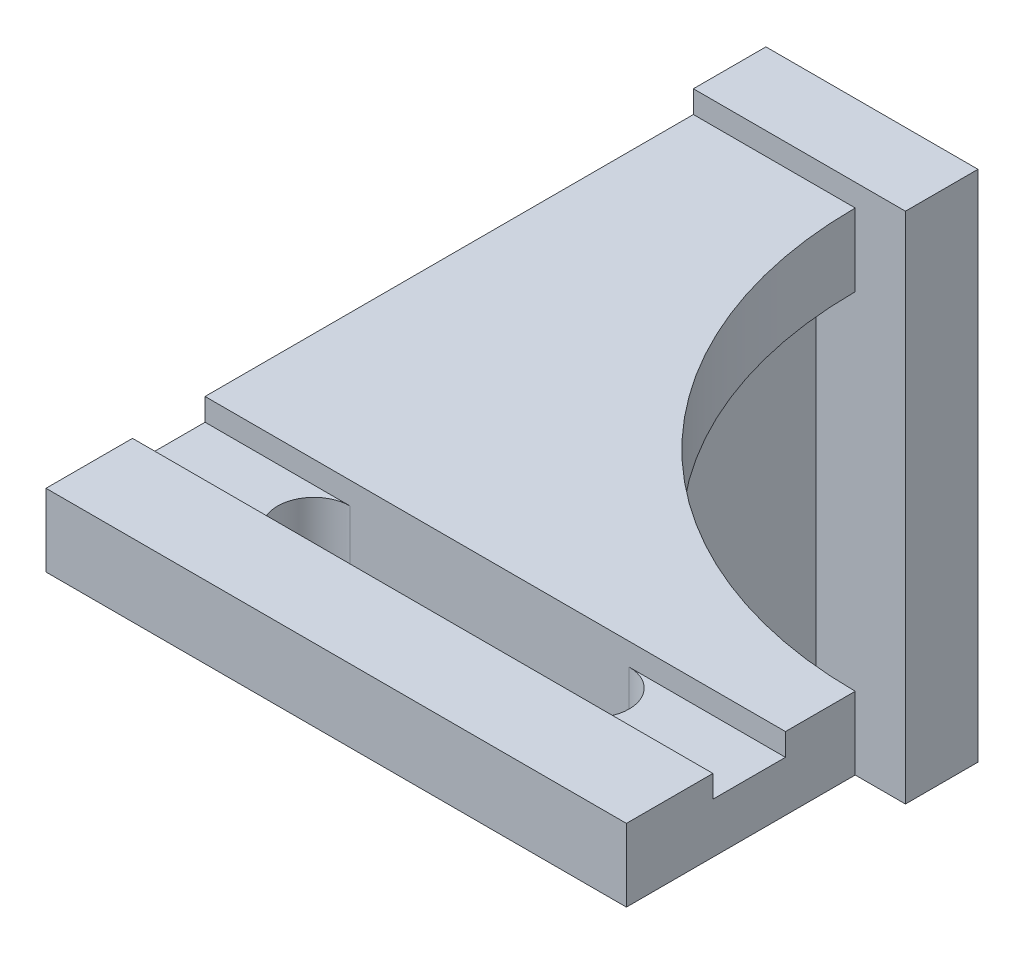
ISO-10303-21;
HEADER;
FILE_DESCRIPTION(('STEP AP214'),'2;1');
FILE_NAME('part.step','',(''),(''),'','','');
FILE_SCHEMA(('AUTOMOTIVE_DESIGN { 1 0 10303 214 1 1 1 1 }'));
ENDSEC;
DATA;
#1=APPLICATION_CONTEXT('core data for automotive mechanical design processes');
#2=APPLICATION_PROTOCOL_DEFINITION('international standard','automotive_design',2000,#1);
#3=PRODUCT_CONTEXT('',#1,'mechanical');
#4=PRODUCT('Part','Part','',(#3));
#5=PRODUCT_RELATED_PRODUCT_CATEGORY('part','',(#4));
#6=PRODUCT_DEFINITION_FORMATION('','',#4);
#7=PRODUCT_DEFINITION_CONTEXT('part definition',#1,'design');
#8=PRODUCT_DEFINITION('design','',#6,#7);
#9=PRODUCT_DEFINITION_SHAPE('','',#8);
#10=(LENGTH_UNIT() NAMED_UNIT(*) SI_UNIT(.MILLI.,.METRE.));
#11=(NAMED_UNIT(*) PLANE_ANGLE_UNIT() SI_UNIT($,.RADIAN.));
#12=(NAMED_UNIT(*) SI_UNIT($,.STERADIAN.) SOLID_ANGLE_UNIT());
#13=UNCERTAINTY_MEASURE_WITH_UNIT(LENGTH_MEASURE(1.E-05),#10,'distance_accuracy_value','');
#14=(GEOMETRIC_REPRESENTATION_CONTEXT(3) GLOBAL_UNCERTAINTY_ASSIGNED_CONTEXT((#13)) GLOBAL_UNIT_ASSIGNED_CONTEXT((#10,
#11,#12)) REPRESENTATION_CONTEXT('',''));
#15=CARTESIAN_POINT('',(0.,0.,0.));
#16=DIRECTION('',(0.,0.,1.));
#17=DIRECTION('',(1.,0.,0.));
#18=AXIS2_PLACEMENT_3D('',#15,#16,#17);
#19=CARTESIAN_POINT('',(38.,-86.,13.));
#20=DIRECTION('',(0.,-0.674269364021332,0.738485493928126));
#21=DIRECTION('',(0.,-0.738485493928126,-0.674269364021332));
#22=AXIS2_PLACEMENT_3D('',#19,#20,#21);
#23=PLANE('',#22);
#24=DIRECTION('',(-1.,0.,0.));
#25=VECTOR('',#24,1.);
#26=CARTESIAN_POINT('',(38.,-17.,76.));
#27=LINE('',#26,#25);
#28=CARTESIAN_POINT('',(22.,-17.,76.));
#29=VERTEX_POINT('',#28);
#30=CARTESIAN_POINT('',(16.,-17.,76.));
#31=VERTEX_POINT('',#30);
#32=EDGE_CURVE('E211',#29,#31,#27,.T.);
#33=ORIENTED_EDGE('',*,*,#32,.T.);
#34=DIRECTION('',(0.,0.738485493928126,0.674269364021332));
#35=VECTOR('',#34,1.);
#36=CARTESIAN_POINT('',(16.,-17.,76.));
#37=LINE('',#36,#35);
#38=CARTESIAN_POINT('',(16.,-86.,13.));
#39=VERTEX_POINT('',#38);
#40=EDGE_CURVE('E196',#39,#31,#37,.T.);
#41=ORIENTED_EDGE('',*,*,#40,.F.);
#42=DIRECTION('',(-1.,0.,0.));
#43=VECTOR('',#42,1.);
#44=CARTESIAN_POINT('',(38.,-86.,13.));
#45=LINE('',#44,#43);
#46=CARTESIAN_POINT('',(22.,-86.,13.));
#47=VERTEX_POINT('',#46);
#48=EDGE_CURVE('E202',#47,#39,#45,.T.);
#49=ORIENTED_EDGE('',*,*,#48,.F.);
#50=DIRECTION('',(0.,-0.738485493928126,-0.674269364021332));
#51=VECTOR('',#50,1.);
#52=CARTESIAN_POINT('',(22.,-86.,13.));
#53=LINE('',#52,#51);
#54=EDGE_CURVE('E193',#29,#47,#53,.T.);
#55=ORIENTED_EDGE('',*,*,#54,.F.);
#56=EDGE_LOOP('',(#33,#41,#49,#55));
#57=FACE_BOUND('',#56,.T.);
#58=ADVANCED_FACE('F44',(#57),#23,.T.);
#59=CARTESIAN_POINT('',(104.,-8.,100.5));
#60=DIRECTION('',(0.,1.,0.));
#61=DIRECTION('',(0.,0.,1.));
#62=AXIS2_PLACEMENT_3D('',#59,#60,#61);
#63=PLANE('',#62);
#64=CARTESIAN_POINT('',(26.,-8.,107.));
#65=DIRECTION('',(0.,1.,0.));
#66=DIRECTION('',(0.,0.,1.));
#67=AXIS2_PLACEMENT_3D('',#64,#65,#66);
#68=CIRCLE('',#67,6.50000000000001);
#69=CARTESIAN_POINT('',(26.,-8.,100.5));
#70=VERTEX_POINT('',#69);
#71=CARTESIAN_POINT('',(26.,-8.,113.5));
#72=VERTEX_POINT('',#71);
#73=EDGE_CURVE('E239',#70,#72,#68,.T.);
#74=ORIENTED_EDGE('',*,*,#73,.F.);
#75=DIRECTION('',(-1.,0.,0.));
#76=VECTOR('',#75,1.);
#77=CARTESIAN_POINT('',(104.,-8.,100.5));
#78=LINE('',#77,#76);
#79=CARTESIAN_POINT('',(0.,-8.,100.5));
#80=VERTEX_POINT('',#79);
#81=EDGE_CURVE('E296',#70,#80,#78,.T.);
#82=ORIENTED_EDGE('',*,*,#81,.T.);
#83=DIRECTION('',(0.,0.,-1.));
#84=VECTOR('',#83,1.);
#85=CARTESIAN_POINT('',(0.,-8.,100.5));
#86=LINE('',#85,#84);
#87=CARTESIAN_POINT('',(0.,-8.,113.5));
#88=VERTEX_POINT('',#87);
#89=EDGE_CURVE('E283',#88,#80,#86,.T.);
#90=ORIENTED_EDGE('',*,*,#89,.F.);
#91=DIRECTION('',(-1.,0.,0.));
#92=VECTOR('',#91,1.);
#93=CARTESIAN_POINT('',(104.,-8.,113.5));
#94=LINE('',#93,#92);
#95=EDGE_CURVE('E305',#72,#88,#94,.T.);
#96=ORIENTED_EDGE('',*,*,#95,.F.);
#97=EDGE_LOOP('',(#74,#82,#90,#96));
#98=FACE_BOUND('',#97,.T.);
#99=ADVANCED_FACE('F374',(#98),#63,.T.);
#100=CARTESIAN_POINT('',(0.,-92.,13.));
#101=DIRECTION('',(1.,0.,0.));
#102=DIRECTION('',(0.,0.,-1.));
#103=AXIS2_PLACEMENT_3D('',#100,#101,#102);
#104=PLANE('',#103);
#105=DIRECTION('',(0.,-1.,0.));
#106=VECTOR('',#105,1.);
#107=CARTESIAN_POINT('',(0.,-92.,13.));
#108=LINE('',#107,#106);
#109=CARTESIAN_POINT('',(0.,-17.,13.));
#110=VERTEX_POINT('',#109);
#111=CARTESIAN_POINT('',(0.,-92.,13.));
#112=VERTEX_POINT('',#111);
#113=EDGE_CURVE('E315',#110,#112,#108,.T.);
#114=ORIENTED_EDGE('',*,*,#113,.F.);
#115=DIRECTION('',(0.,0.,1.));
#116=VECTOR('',#115,1.);
#117=CARTESIAN_POINT('',(0.,-17.,129.));
#118=LINE('',#117,#116);
#119=CARTESIAN_POINT('',(0.,-17.,129.));
#120=VERTEX_POINT('',#119);
#121=EDGE_CURVE('E195',#110,#120,#118,.T.);
#122=ORIENTED_EDGE('',*,*,#121,.T.);
#123=DIRECTION('',(0.,1.,0.));
#124=VECTOR('',#123,1.);
#125=CARTESIAN_POINT('',(0.,-4.,129.));
#126=LINE('',#125,#124);
#127=CARTESIAN_POINT('',(0.,-4.,129.));
#128=VERTEX_POINT('',#127);
#129=EDGE_CURVE('E273',#120,#128,#126,.T.);
#130=ORIENTED_EDGE('',*,*,#129,.T.);
#131=DIRECTION('',(0.,0.,-1.));
#132=VECTOR('',#131,1.);
#133=CARTESIAN_POINT('',(0.,-4.,113.5));
#134=LINE('',#133,#132);
#135=CARTESIAN_POINT('',(0.,-4.,113.5));
#136=VERTEX_POINT('',#135);
#137=EDGE_CURVE('E279',#128,#136,#134,.T.);
#138=ORIENTED_EDGE('',*,*,#137,.T.);
#139=DIRECTION('',(0.,-1.,0.));
#140=VECTOR('',#139,1.);
#141=CARTESIAN_POINT('',(0.,-8.,113.5));
#142=LINE('',#141,#140);
#143=EDGE_CURVE('E281',#136,#88,#142,.T.);
#144=ORIENTED_EDGE('',*,*,#143,.T.);
#145=ORIENTED_EDGE('',*,*,#89,.T.);
#146=DIRECTION('',(0.,1.,0.));
#147=VECTOR('',#146,1.);
#148=CARTESIAN_POINT('',(0.,-4.,100.5));
#149=LINE('',#148,#147);
#150=CARTESIAN_POINT('',(0.,-4.,100.5));
#151=VERTEX_POINT('',#150);
#152=EDGE_CURVE('E290',#80,#151,#149,.T.);
#153=ORIENTED_EDGE('',*,*,#152,.T.);
#154=DIRECTION('',(0.,0.,-1.));
#155=VECTOR('',#154,1.);
#156=CARTESIAN_POINT('',(0.,-4.,13.));
#157=LINE('',#156,#155);
#158=CARTESIAN_POINT('',(0.,-4.,13.));
#159=VERTEX_POINT('',#158);
#160=EDGE_CURVE('E253',#151,#159,#157,.T.);
#161=ORIENTED_EDGE('',*,*,#160,.T.);
#162=CARTESIAN_POINT('',(0.,0.,13.));
#163=VERTEX_POINT('',#162);
#164=EDGE_CURVE('E308',#163,#159,#108,.T.);
#165=ORIENTED_EDGE('',*,*,#164,.F.);
#166=DIRECTION('',(0.,0.,-1.));
#167=VECTOR('',#166,1.);
#168=CARTESIAN_POINT('',(0.,0.,13.));
#169=LINE('',#168,#167);
#170=CARTESIAN_POINT('',(0.,0.,0.));
#171=VERTEX_POINT('',#170);
#172=EDGE_CURVE('E319',#163,#171,#169,.T.);
#173=ORIENTED_EDGE('',*,*,#172,.T.);
#174=DIRECTION('',(0.,-1.,0.));
#175=VECTOR('',#174,1.);
#176=CARTESIAN_POINT('',(0.,-92.,0.));
#177=LINE('',#176,#175);
#178=CARTESIAN_POINT('',(0.,-92.,0.));
#179=VERTEX_POINT('',#178);
#180=EDGE_CURVE('E295',#171,#179,#177,.T.);
#181=ORIENTED_EDGE('',*,*,#180,.T.);
#182=DIRECTION('',(0.,0.,-1.));
#183=VECTOR('',#182,1.);
#184=CARTESIAN_POINT('',(0.,-92.,13.));
#185=LINE('',#184,#183);
#186=EDGE_CURVE('E47',#112,#179,#185,.T.);
#187=ORIENTED_EDGE('',*,*,#186,.F.);
#188=EDGE_LOOP('',(#114,#122,#130,#138,#144,#145,#153,#161,#165,#173,#181,#187));
#189=FACE_BOUND('',#188,.T.);
#190=ADVANCED_FACE('F50',(#189),#104,.F.);
#191=CARTESIAN_POINT('',(38.,-92.,13.));
#192=DIRECTION('',(0.,1.,0.));
#193=DIRECTION('',(0.,0.,1.));
#194=AXIS2_PLACEMENT_3D('',#191,#192,#193);
#195=PLANE('',#194);
#196=DIRECTION('',(1.,0.,0.));
#197=VECTOR('',#196,1.);
#198=CARTESIAN_POINT('',(38.,-92.,0.));
#199=LINE('',#198,#197);
#200=CARTESIAN_POINT('',(38.,-92.,0.));
#201=VERTEX_POINT('',#200);
#202=EDGE_CURVE('E322',#179,#201,#199,.T.);
#203=ORIENTED_EDGE('',*,*,#202,.T.);
#204=DIRECTION('',(0.,0.,-1.));
#205=VECTOR('',#204,1.);
#206=CARTESIAN_POINT('',(38.,-92.,13.));
#207=LINE('',#206,#205);
#208=CARTESIAN_POINT('',(38.,-92.,13.));
#209=VERTEX_POINT('',#208);
#210=EDGE_CURVE('E332',#209,#201,#207,.T.);
#211=ORIENTED_EDGE('',*,*,#210,.F.);
#212=DIRECTION('',(1.,0.,0.));
#213=VECTOR('',#212,1.);
#214=CARTESIAN_POINT('',(38.,-92.,13.));
#215=LINE('',#214,#213);
#216=EDGE_CURVE('E311',#112,#209,#215,.T.);
#217=ORIENTED_EDGE('',*,*,#216,.F.);
#218=ORIENTED_EDGE('',*,*,#186,.T.);
#219=EDGE_LOOP('',(#203,#211,#217,#218));
#220=FACE_BOUND('',#219,.T.);
#221=ADVANCED_FACE('F342',(#220),#195,.F.);
#222=CARTESIAN_POINT('',(38.,0.,13.));
#223=DIRECTION('',(-1.,0.,0.));
#224=DIRECTION('',(0.,0.,1.));
#225=AXIS2_PLACEMENT_3D('',#222,#223,#224);
#226=PLANE('',#225);
#227=DIRECTION('',(0.,0.,-1.));
#228=VECTOR('',#227,1.);
#229=CARTESIAN_POINT('',(38.,0.,13.));
#230=LINE('',#229,#228);
#231=CARTESIAN_POINT('',(38.,0.,13.));
#232=VERTEX_POINT('',#231);
#233=CARTESIAN_POINT('',(38.,0.,0.));
#234=VERTEX_POINT('',#233);
#235=EDGE_CURVE('E328',#232,#234,#230,.T.);
#236=ORIENTED_EDGE('',*,*,#235,.F.);
#237=DIRECTION('',(0.,1.,0.));
#238=VECTOR('',#237,1.);
#239=CARTESIAN_POINT('',(38.,0.,13.));
#240=LINE('',#239,#238);
#241=EDGE_CURVE('E313',#209,#232,#240,.T.);
#242=ORIENTED_EDGE('',*,*,#241,.F.);
#243=ORIENTED_EDGE('',*,*,#210,.T.);
#244=DIRECTION('',(0.,1.,0.));
#245=VECTOR('',#244,1.);
#246=CARTESIAN_POINT('',(38.,0.,0.));
#247=LINE('',#246,#245);
#248=EDGE_CURVE('E324',#201,#234,#247,.T.);
#249=ORIENTED_EDGE('',*,*,#248,.T.);
#250=EDGE_LOOP('',(#236,#242,#243,#249));
#251=FACE_BOUND('',#250,.T.);
#252=ADVANCED_FACE('F350',(#251),#226,.F.);
#253=CARTESIAN_POINT('',(0.,0.,13.));
#254=DIRECTION('',(0.,-1.,0.));
#255=DIRECTION('',(0.,0.,-1.));
#256=AXIS2_PLACEMENT_3D('',#253,#254,#255);
#257=PLANE('',#256);
#258=DIRECTION('',(-1.,0.,0.));
#259=VECTOR('',#258,1.);
#260=CARTESIAN_POINT('',(0.,0.,0.));
#261=LINE('',#260,#259);
#262=EDGE_CURVE('E323',#234,#171,#261,.T.);
#263=ORIENTED_EDGE('',*,*,#262,.T.);
#264=ORIENTED_EDGE('',*,*,#172,.F.);
#265=DIRECTION('',(-1.,0.,0.));
#266=VECTOR('',#265,1.);
#267=CARTESIAN_POINT('',(0.,0.,13.));
#268=LINE('',#267,#266);
#269=EDGE_CURVE('E317',#232,#163,#268,.T.);
#270=ORIENTED_EDGE('',*,*,#269,.F.);
#271=ORIENTED_EDGE('',*,*,#235,.T.);
#272=EDGE_LOOP('',(#263,#264,#270,#271));
#273=FACE_BOUND('',#272,.T.);
#274=ADVANCED_FACE('F353',(#273),#257,.F.);
#275=CARTESIAN_POINT('',(0.,0.,13.));
#276=DIRECTION('',(0.,0.,-1.));
#277=DIRECTION('',(-1.,0.,0.));
#278=AXIS2_PLACEMENT_3D('',#275,#276,#277);
#279=PLANE('',#278);
#280=ORIENTED_EDGE('',*,*,#241,.T.);
#281=ORIENTED_EDGE('',*,*,#269,.T.);
#282=ORIENTED_EDGE('',*,*,#164,.T.);
#283=DIRECTION('',(-1.,0.,0.));
#284=VECTOR('',#283,1.);
#285=CARTESIAN_POINT('',(104.,-4.,13.));
#286=LINE('',#285,#284);
#287=CARTESIAN_POINT('',(29.,-4.,13.));
#288=VERTEX_POINT('',#287);
#289=EDGE_CURVE('E11',#288,#159,#286,.T.);
#290=ORIENTED_EDGE('',*,*,#289,.F.);
#291=DIRECTION('',(0.,-1.,0.));
#292=VECTOR('',#291,1.);
#293=CARTESIAN_POINT('',(29.,-4.,13.));
#294=LINE('',#293,#292);
#295=CARTESIAN_POINT('',(29.,-17.,13.));
#296=VERTEX_POINT('',#295);
#297=EDGE_CURVE('E247',#288,#296,#294,.T.);
#298=ORIENTED_EDGE('',*,*,#297,.T.);
#299=DIRECTION('',(1.,0.,0.));
#300=VECTOR('',#299,1.);
#301=CARTESIAN_POINT('',(22.,-17.,13.));
#302=LINE('',#301,#300);
#303=CARTESIAN_POINT('',(22.,-17.,13.));
#304=VERTEX_POINT('',#303);
#305=EDGE_CURVE('E215',#304,#296,#302,.T.);
#306=ORIENTED_EDGE('',*,*,#305,.F.);
#307=DIRECTION('',(0.,1.,0.));
#308=VECTOR('',#307,1.);
#309=CARTESIAN_POINT('',(22.,-17.,13.));
#310=LINE('',#309,#308);
#311=EDGE_CURVE('E209',#47,#304,#310,.T.);
#312=ORIENTED_EDGE('',*,*,#311,.F.);
#313=ORIENTED_EDGE('',*,*,#48,.T.);
#314=DIRECTION('',(0.,-1.,0.));
#315=VECTOR('',#314,1.);
#316=CARTESIAN_POINT('',(16.,-86.,13.));
#317=LINE('',#316,#315);
#318=CARTESIAN_POINT('',(16.,-17.,13.));
#319=VERTEX_POINT('',#318);
#320=EDGE_CURVE('E62',#319,#39,#317,.T.);
#321=ORIENTED_EDGE('',*,*,#320,.F.);
#322=DIRECTION('',(-1.,0.,0.));
#323=VECTOR('',#322,1.);
#324=CARTESIAN_POINT('',(16.,-17.,13.));
#325=LINE('',#324,#323);
#326=EDGE_CURVE('E184',#319,#110,#325,.T.);
#327=ORIENTED_EDGE('',*,*,#326,.T.);
#328=ORIENTED_EDGE('',*,*,#113,.T.);
#329=ORIENTED_EDGE('',*,*,#216,.T.);
#330=EDGE_LOOP('',(#280,#281,#282,#290,#298,#306,#312,#313,#321,#327,#328,#329));
#331=FACE_BOUND('',#330,.T.);
#332=ADVANCED_FACE('F198',(#331),#279,.F.);
#333=CARTESIAN_POINT('',(0.,0.,0.));
#334=DIRECTION('',(0.,0.,-1.));
#335=DIRECTION('',(-1.,0.,0.));
#336=AXIS2_PLACEMENT_3D('',#333,#334,#335);
#337=PLANE('',#336);
#338=ORIENTED_EDGE('',*,*,#180,.F.);
#339=ORIENTED_EDGE('',*,*,#262,.F.);
#340=ORIENTED_EDGE('',*,*,#248,.F.);
#341=ORIENTED_EDGE('',*,*,#202,.F.);
#342=EDGE_LOOP('',(#338,#339,#340,#341));
#343=FACE_BOUND('',#342,.T.);
#344=ADVANCED_FACE('F349',(#343),#337,.T.);
#345=CARTESIAN_POINT('',(104.,-4.,13.));
#346=DIRECTION('',(0.,1.,0.));
#347=DIRECTION('',(0.,0.,1.));
#348=AXIS2_PLACEMENT_3D('',#345,#346,#347);
#349=PLANE('',#348);
#350=CARTESIAN_POINT('',(104.,-4.,13.));
#351=DIRECTION('',(0.,-1.,0.));
#352=DIRECTION('',(0.,0.,-1.));
#353=AXIS2_PLACEMENT_3D('',#350,#351,#352);
#354=CIRCLE('',#353,75.);
#355=CARTESIAN_POINT('',(104.,-4.,88.));
#356=VERTEX_POINT('',#355);
#357=EDGE_CURVE('E243',#356,#288,#354,.T.);
#358=ORIENTED_EDGE('',*,*,#357,.T.);
#359=ORIENTED_EDGE('',*,*,#289,.T.);
#360=ORIENTED_EDGE('',*,*,#160,.F.);
#361=DIRECTION('',(-1.,0.,0.));
#362=VECTOR('',#361,1.);
#363=CARTESIAN_POINT('',(104.,-4.,100.5));
#364=LINE('',#363,#362);
#365=CARTESIAN_POINT('',(104.,-4.,100.5));
#366=VERTEX_POINT('',#365);
#367=EDGE_CURVE('E292',#366,#151,#364,.T.);
#368=ORIENTED_EDGE('',*,*,#367,.F.);
#369=DIRECTION('',(0.,0.,-1.));
#370=VECTOR('',#369,1.);
#371=CARTESIAN_POINT('',(104.,-4.,13.));
#372=LINE('',#371,#370);
#373=EDGE_CURVE('E266',#366,#356,#372,.T.);
#374=ORIENTED_EDGE('',*,*,#373,.T.);
#375=EDGE_LOOP('',(#358,#359,#360,#368,#374));
#376=FACE_BOUND('',#375,.T.);
#377=ADVANCED_FACE('F385',(#376),#349,.T.);
#378=CARTESIAN_POINT('',(104.,-4.,100.5));
#379=DIRECTION('',(0.,0.,1.));
#380=DIRECTION('',(1.,0.,0.));
#381=AXIS2_PLACEMENT_3D('',#378,#379,#380);
#382=PLANE('',#381);
#383=ORIENTED_EDGE('',*,*,#81,.F.);
#384=DIRECTION('',(0.,-1.,0.));
#385=VECTOR('',#384,1.);
#386=CARTESIAN_POINT('',(26.,-4.,100.5));
#387=LINE('',#386,#385);
#388=CARTESIAN_POINT('',(26.,-17.,100.5));
#389=VERTEX_POINT('',#388);
#390=EDGE_CURVE('E226',#70,#389,#387,.T.);
#391=ORIENTED_EDGE('',*,*,#390,.T.);
#392=DIRECTION('',(1.,0.,0.));
#393=VECTOR('',#392,1.);
#394=CARTESIAN_POINT('',(26.,-17.,100.5));
#395=LINE('',#394,#393);
#396=CARTESIAN_POINT('',(76.,-17.,100.5));
#397=VERTEX_POINT('',#396);
#398=EDGE_CURVE('E218',#389,#397,#395,.T.);
#399=ORIENTED_EDGE('',*,*,#398,.T.);
#400=DIRECTION('',(0.,-1.,0.));
#401=VECTOR('',#400,1.);
#402=CARTESIAN_POINT('',(76.,-4.,100.5));
#403=LINE('',#402,#401);
#404=CARTESIAN_POINT('',(76.,-8.,100.5));
#405=VERTEX_POINT('',#404);
#406=EDGE_CURVE('E234',#405,#397,#403,.T.);
#407=ORIENTED_EDGE('',*,*,#406,.F.);
#408=CARTESIAN_POINT('',(104.,-8.,100.5));
#409=VERTEX_POINT('',#408);
#410=EDGE_CURVE('E294',#409,#405,#78,.T.);
#411=ORIENTED_EDGE('',*,*,#410,.F.);
#412=DIRECTION('',(0.,1.,0.));
#413=VECTOR('',#412,1.);
#414=CARTESIAN_POINT('',(104.,-4.,100.5));
#415=LINE('',#414,#413);
#416=EDGE_CURVE('E270',#409,#366,#415,.T.);
#417=ORIENTED_EDGE('',*,*,#416,.T.);
#418=ORIENTED_EDGE('',*,*,#367,.T.);
#419=ORIENTED_EDGE('',*,*,#152,.F.);
#420=EDGE_LOOP('',(#383,#391,#399,#407,#411,#417,#418,#419));
#421=FACE_BOUND('',#420,.T.);
#422=ADVANCED_FACE('F378',(#421),#382,.T.);
#423=CARTESIAN_POINT('',(76.,-8.,107.));
#424=DIRECTION('',(0.,1.,0.));
#425=DIRECTION('',(0.,0.,1.));
#426=AXIS2_PLACEMENT_3D('',#423,#424,#425);
#427=CIRCLE('',#426,6.50000000000001);
#428=CARTESIAN_POINT('',(76.,-8.,113.5));
#429=VERTEX_POINT('',#428);
#430=EDGE_CURVE('E233',#429,#405,#427,.T.);
#431=ORIENTED_EDGE('',*,*,#430,.F.);
#432=CARTESIAN_POINT('',(104.,-8.,113.5));
#433=VERTEX_POINT('',#432);
#434=EDGE_CURVE('E299',#433,#429,#94,.T.);
#435=ORIENTED_EDGE('',*,*,#434,.F.);
#436=DIRECTION('',(0.,0.,-1.));
#437=VECTOR('',#436,1.);
#438=CARTESIAN_POINT('',(104.,-8.,100.5));
#439=LINE('',#438,#437);
#440=EDGE_CURVE('E263',#433,#409,#439,.T.);
#441=ORIENTED_EDGE('',*,*,#440,.T.);
#442=ORIENTED_EDGE('',*,*,#410,.T.);
#443=EDGE_LOOP('',(#431,#435,#441,#442));
#444=FACE_BOUND('',#443,.T.);
#445=ADVANCED_FACE('F403',(#444),#63,.T.);
#446=CARTESIAN_POINT('',(104.,-8.,113.5));
#447=DIRECTION('',(0.,0.,-1.));
#448=DIRECTION('',(-1.,0.,0.));
#449=AXIS2_PLACEMENT_3D('',#446,#447,#448);
#450=PLANE('',#449);
#451=ORIENTED_EDGE('',*,*,#434,.T.);
#452=DIRECTION('',(0.,-1.,0.));
#453=VECTOR('',#452,1.);
#454=CARTESIAN_POINT('',(76.,-4.,113.5));
#455=LINE('',#454,#453);
#456=CARTESIAN_POINT('',(76.,-17.,113.5));
#457=VERTEX_POINT('',#456);
#458=EDGE_CURVE('E235',#429,#457,#455,.T.);
#459=ORIENTED_EDGE('',*,*,#458,.T.);
#460=DIRECTION('',(-1.,0.,0.));
#461=VECTOR('',#460,1.);
#462=CARTESIAN_POINT('',(26.,-17.,113.5));
#463=LINE('',#462,#461);
#464=CARTESIAN_POINT('',(26.,-17.,113.5));
#465=VERTEX_POINT('',#464);
#466=EDGE_CURVE('E221',#457,#465,#463,.T.);
#467=ORIENTED_EDGE('',*,*,#466,.T.);
#468=DIRECTION('',(0.,-1.,0.));
#469=VECTOR('',#468,1.);
#470=CARTESIAN_POINT('',(26.,-4.,113.5));
#471=LINE('',#470,#469);
#472=EDGE_CURVE('E230',#72,#465,#471,.T.);
#473=ORIENTED_EDGE('',*,*,#472,.F.);
#474=ORIENTED_EDGE('',*,*,#95,.T.);
#475=ORIENTED_EDGE('',*,*,#143,.F.);
#476=DIRECTION('',(-1.,0.,0.));
#477=VECTOR('',#476,1.);
#478=CARTESIAN_POINT('',(104.,-4.,113.5));
#479=LINE('',#478,#477);
#480=CARTESIAN_POINT('',(104.,-4.,113.5));
#481=VERTEX_POINT('',#480);
#482=EDGE_CURVE('E303',#481,#136,#479,.T.);
#483=ORIENTED_EDGE('',*,*,#482,.F.);
#484=DIRECTION('',(0.,-1.,0.));
#485=VECTOR('',#484,1.);
#486=CARTESIAN_POINT('',(104.,-8.,113.5));
#487=LINE('',#486,#485);
#488=EDGE_CURVE('E261',#481,#433,#487,.T.);
#489=ORIENTED_EDGE('',*,*,#488,.T.);
#490=EDGE_LOOP('',(#451,#459,#467,#473,#474,#475,#483,#489));
#491=FACE_BOUND('',#490,.T.);
#492=ADVANCED_FACE('F367',(#491),#450,.T.);
#493=CARTESIAN_POINT('',(104.,-4.,113.5));
#494=DIRECTION('',(0.,1.,0.));
#495=DIRECTION('',(0.,0.,1.));
#496=AXIS2_PLACEMENT_3D('',#493,#494,#495);
#497=PLANE('',#496);
#498=ORIENTED_EDGE('',*,*,#137,.F.);
#499=DIRECTION('',(-1.,0.,0.));
#500=VECTOR('',#499,1.);
#501=CARTESIAN_POINT('',(104.,-4.,129.));
#502=LINE('',#501,#500);
#503=CARTESIAN_POINT('',(104.,-4.,129.));
#504=VERTEX_POINT('',#503);
#505=EDGE_CURVE('E304',#504,#128,#502,.T.);
#506=ORIENTED_EDGE('',*,*,#505,.F.);
#507=DIRECTION('',(0.,0.,-1.));
#508=VECTOR('',#507,1.);
#509=CARTESIAN_POINT('',(104.,-4.,113.5));
#510=LINE('',#509,#508);
#511=EDGE_CURVE('E259',#504,#481,#510,.T.);
#512=ORIENTED_EDGE('',*,*,#511,.T.);
#513=ORIENTED_EDGE('',*,*,#482,.T.);
#514=EDGE_LOOP('',(#498,#506,#512,#513));
#515=FACE_BOUND('',#514,.T.);
#516=ADVANCED_FACE('F362',(#515),#497,.T.);
#517=CARTESIAN_POINT('',(104.,-4.,129.));
#518=DIRECTION('',(0.,0.,1.));
#519=DIRECTION('',(1.,0.,0.));
#520=AXIS2_PLACEMENT_3D('',#517,#518,#519);
#521=PLANE('',#520);
#522=ORIENTED_EDGE('',*,*,#129,.F.);
#523=DIRECTION('',(-1.,0.,0.));
#524=VECTOR('',#523,1.);
#525=CARTESIAN_POINT('',(104.,-17.,129.));
#526=LINE('',#525,#524);
#527=CARTESIAN_POINT('',(104.,-17.,129.));
#528=VERTEX_POINT('',#527);
#529=EDGE_CURVE('E271',#528,#120,#526,.T.);
#530=ORIENTED_EDGE('',*,*,#529,.F.);
#531=DIRECTION('',(0.,1.,0.));
#532=VECTOR('',#531,1.);
#533=CARTESIAN_POINT('',(104.,-4.,129.));
#534=LINE('',#533,#532);
#535=EDGE_CURVE('E251',#528,#504,#534,.T.);
#536=ORIENTED_EDGE('',*,*,#535,.T.);
#537=ORIENTED_EDGE('',*,*,#505,.T.);
#538=EDGE_LOOP('',(#522,#530,#536,#537));
#539=FACE_BOUND('',#538,.T.);
#540=ADVANCED_FACE('F363',(#539),#521,.T.);
#541=CARTESIAN_POINT('',(104.,-17.,129.));
#542=DIRECTION('',(0.,-1.,0.));
#543=DIRECTION('',(0.,0.,-1.));
#544=AXIS2_PLACEMENT_3D('',#541,#542,#543);
#545=PLANE('',#544);
#546=ORIENTED_EDGE('',*,*,#305,.T.);
#547=CARTESIAN_POINT('',(104.,-17.,13.));
#548=DIRECTION('',(0.,-1.,0.));
#549=DIRECTION('',(0.,0.,-1.));
#550=AXIS2_PLACEMENT_3D('',#547,#548,#549);
#551=CIRCLE('',#550,75.);
#552=CARTESIAN_POINT('',(104.,-17.,88.));
#553=VERTEX_POINT('',#552);
#554=EDGE_CURVE('E245',#553,#296,#551,.T.);
#555=ORIENTED_EDGE('',*,*,#554,.F.);
#556=DIRECTION('',(0.,0.,1.));
#557=VECTOR('',#556,1.);
#558=CARTESIAN_POINT('',(104.,-17.,129.));
#559=LINE('',#558,#557);
#560=EDGE_CURVE('E255',#553,#528,#559,.T.);
#561=ORIENTED_EDGE('',*,*,#560,.T.);
#562=ORIENTED_EDGE('',*,*,#529,.T.);
#563=ORIENTED_EDGE('',*,*,#121,.F.);
#564=ORIENTED_EDGE('',*,*,#326,.F.);
#565=DIRECTION('',(0.,0.,-1.));
#566=VECTOR('',#565,1.);
#567=CARTESIAN_POINT('',(16.,-17.,13.));
#568=LINE('',#567,#566);
#569=EDGE_CURVE('E188',#31,#319,#568,.T.);
#570=ORIENTED_EDGE('',*,*,#569,.F.);
#571=ORIENTED_EDGE('',*,*,#32,.F.);
#572=DIRECTION('',(0.,0.,1.));
#573=VECTOR('',#572,1.);
#574=CARTESIAN_POINT('',(22.,-17.,76.));
#575=LINE('',#574,#573);
#576=EDGE_CURVE('E68',#304,#29,#575,.T.);
#577=ORIENTED_EDGE('',*,*,#576,.F.);
#578=EDGE_LOOP('',(#546,#555,#561,#562,#563,#564,#570,#571,#577));
#579=FACE_BOUND('',#578,.T.);
#580=CARTESIAN_POINT('',(26.,-17.,107.));
#581=DIRECTION('',(0.,-1.,0.));
#582=DIRECTION('',(0.,0.,-1.));
#583=AXIS2_PLACEMENT_3D('',#580,#581,#582);
#584=CIRCLE('',#583,6.50000000000001);
#585=EDGE_CURVE('E216',#465,#389,#584,.T.);
#586=ORIENTED_EDGE('',*,*,#585,.F.);
#587=ORIENTED_EDGE('',*,*,#466,.F.);
#588=CARTESIAN_POINT('',(76.,-17.,107.));
#589=DIRECTION('',(0.,-1.,0.));
#590=DIRECTION('',(0.,0.,-1.));
#591=AXIS2_PLACEMENT_3D('',#588,#589,#590);
#592=CIRCLE('',#591,6.50000000000001);
#593=EDGE_CURVE('E225',#397,#457,#592,.T.);
#594=ORIENTED_EDGE('',*,*,#593,.F.);
#595=ORIENTED_EDGE('',*,*,#398,.F.);
#596=EDGE_LOOP('',(#586,#587,#594,#595));
#597=FACE_BOUND('',#596,.T.);
#598=ADVANCED_FACE('F190',(#579,#597),#545,.T.);
#599=CARTESIAN_POINT('',(104.,0.,0.));
#600=DIRECTION('',(1.,0.,0.));
#601=DIRECTION('',(0.,0.,-1.));
#602=AXIS2_PLACEMENT_3D('',#599,#600,#601);
#603=PLANE('',#602);
#604=DIRECTION('',(0.,-1.,0.));
#605=VECTOR('',#604,1.);
#606=CARTESIAN_POINT('',(104.,-4.,88.));
#607=LINE('',#606,#605);
#608=EDGE_CURVE('E246',#356,#553,#607,.T.);
#609=ORIENTED_EDGE('',*,*,#608,.F.);
#610=ORIENTED_EDGE('',*,*,#373,.F.);
#611=ORIENTED_EDGE('',*,*,#416,.F.);
#612=ORIENTED_EDGE('',*,*,#440,.F.);
#613=ORIENTED_EDGE('',*,*,#488,.F.);
#614=ORIENTED_EDGE('',*,*,#511,.F.);
#615=ORIENTED_EDGE('',*,*,#535,.F.);
#616=ORIENTED_EDGE('',*,*,#560,.F.);
#617=EDGE_LOOP('',(#609,#610,#611,#612,#613,#614,#615,#616));
#618=FACE_BOUND('',#617,.T.);
#619=ADVANCED_FACE('F412',(#618),#603,.T.);
#620=CARTESIAN_POINT('',(104.,-4.,13.));
#621=DIRECTION('',(0.,-1.,0.));
#622=DIRECTION('',(0.,0.,-1.));
#623=AXIS2_PLACEMENT_3D('',#620,#621,#622);
#624=CYLINDRICAL_SURFACE('',#623,75.);
#625=ORIENTED_EDGE('',*,*,#554,.T.);
#626=ORIENTED_EDGE('',*,*,#297,.F.);
#627=ORIENTED_EDGE('',*,*,#357,.F.);
#628=ORIENTED_EDGE('',*,*,#608,.T.);
#629=EDGE_LOOP('',(#625,#626,#627,#628));
#630=FACE_BOUND('',#629,.T.);
#631=ADVANCED_FACE('F381',(#630),#624,.F.);
#632=CARTESIAN_POINT('',(26.,-4.,107.));
#633=DIRECTION('',(0.,-1.,0.));
#634=DIRECTION('',(0.,0.,-1.));
#635=AXIS2_PLACEMENT_3D('',#632,#633,#634);
#636=CYLINDRICAL_SURFACE('',#635,6.50000000000001);
#637=ORIENTED_EDGE('',*,*,#73,.T.);
#638=ORIENTED_EDGE('',*,*,#472,.T.);
#639=ORIENTED_EDGE('',*,*,#585,.T.);
#640=ORIENTED_EDGE('',*,*,#390,.F.);
#641=EDGE_LOOP('',(#637,#638,#639,#640));
#642=FACE_BOUND('',#641,.T.);
#643=ADVANCED_FACE('F397',(#642),#636,.F.);
#644=CARTESIAN_POINT('',(76.,-4.,107.));
#645=DIRECTION('',(0.,-1.,0.));
#646=DIRECTION('',(0.,0.,-1.));
#647=AXIS2_PLACEMENT_3D('',#644,#645,#646);
#648=CYLINDRICAL_SURFACE('',#647,6.50000000000001);
#649=ORIENTED_EDGE('',*,*,#430,.T.);
#650=ORIENTED_EDGE('',*,*,#406,.T.);
#651=ORIENTED_EDGE('',*,*,#593,.T.);
#652=ORIENTED_EDGE('',*,*,#458,.F.);
#653=EDGE_LOOP('',(#649,#650,#651,#652));
#654=FACE_BOUND('',#653,.T.);
#655=ADVANCED_FACE('F386',(#654),#648,.F.);
#656=CARTESIAN_POINT('',(22.,0.,0.));
#657=DIRECTION('',(-1.,0.,0.));
#658=DIRECTION('',(0.,0.,1.));
#659=AXIS2_PLACEMENT_3D('',#656,#657,#658);
#660=PLANE('',#659);
#661=ORIENTED_EDGE('',*,*,#54,.T.);
#662=ORIENTED_EDGE('',*,*,#311,.T.);
#663=ORIENTED_EDGE('',*,*,#576,.T.);
#664=EDGE_LOOP('',(#661,#662,#663));
#665=FACE_BOUND('',#664,.T.);
#666=ADVANCED_FACE('F390',(#665),#660,.F.);
#667=CARTESIAN_POINT('',(16.,0.,0.));
#668=DIRECTION('',(-1.,0.,0.));
#669=DIRECTION('',(0.,0.,1.));
#670=AXIS2_PLACEMENT_3D('',#667,#668,#669);
#671=PLANE('',#670);
#672=ORIENTED_EDGE('',*,*,#569,.T.);
#673=ORIENTED_EDGE('',*,*,#320,.T.);
#674=ORIENTED_EDGE('',*,*,#40,.T.);
#675=EDGE_LOOP('',(#672,#673,#674));
#676=FACE_BOUND('',#675,.T.);
#677=ADVANCED_FACE('F203',(#676),#671,.T.);
#678=CLOSED_SHELL('',(#58,#99,#190,#221,#252,#274,#332,#344,#377,#422,#445,#492,#516,#540,#598,
#619,#631,#643,#655,#666,#677));
#679=MANIFOLD_SOLID_BREP('B2',#678);
#680=ADVANCED_BREP_SHAPE_REPRESENTATION('',(#18,#679),#14);
#681=SHAPE_DEFINITION_REPRESENTATION(#9,#680);
ENDSEC;
END-ISO-10303-21;
